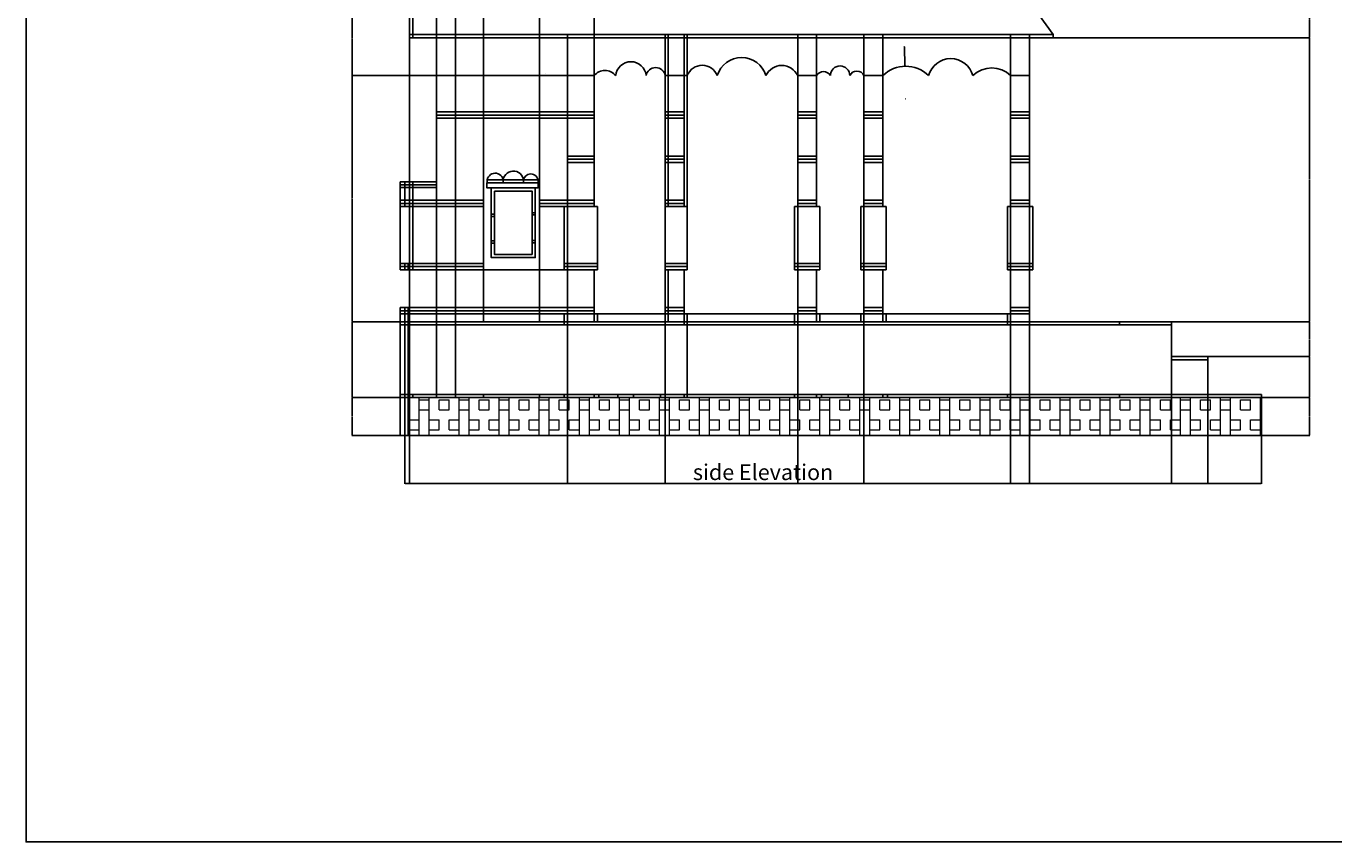
# Model space of a CAD drawing. Units: inches. Extents: x 386 to 107067, y -7 to 96314.
# Tile 1 of 10: x 386 to 1215, y -7 to 510. Entities that reach past the tile are written whole.
import ezdxf

# ---------------------------------------------------------------- set-up
doc = ezdxf.new("R2010")
doc.units = ezdxf.units.IN
for name, color, linetype, lineweight in [('A-ANNO-DIMS', 2, 'Continuous', 18), ('A-ANNO-TEXT', 7, 'Continuous', 25), ('A-ELEV', 7, 'Continuous', 25), ('A-ELEV-PATT', 8, 'Continuous', 13)]:
    doc.layers.add(name, color=color, linetype=linetype, lineweight=lineweight)
doc.styles.get("Standard").update_dxf_attribs({"font": 'arial.ttf'})
doc.dimstyles.get("Standard").update_dxf_attribs({"dimtxt": 0.18, "dimasz": 0.18, "dimexe": 0.18, "dimexo": 0.0625, "dimgap": 0.09, "dimtad": 0, "dimtih": 1, "dimtoh": 1, "dimdec": 4, "dimzin": 0, "dimdsep": 46, "dimtxsty": 'Standard', "dimcen": 0.09, "dimadec": 0, "dimazin": 0, "dimtfac": 1, "dimtdec": 4, "dimtofl": 0, "dimtmove": 0, "dimatfit": 3, "dimfxl": 1, "dimtolj": 1, "dimtzin": 0, "dimarcsym": 0})

# ---------------------------------------------------------------- blocks, each defined once
blk = doc.blocks.new('*D52')
at = {"layer": 'A-ANNO-DIMS', "color": 0, "lineweight": -2, "transparency": 16777216}
for p, q in [((626.03, 250.45), (626.03, 219.83)), ((1169.03, 250.45), (1169.03, 219.83)), ((626.21, 220.01), (897.24, 220.01)), ((1168.85, 220.01), (897.81, 220.01))]:
    blk.add_line(p, q, dxfattribs=at)
at = {"layer": 'A-ANNO-DIMS', "color": 0, "transparency": 16777216}
for points in [[(626.21, 220.04), (626.21, 219.98), (626.03, 220.01)], [(1168.85, 220.04), (1168.85, 219.98), (1169.03, 220.01)]]:
    blk.add_solid(points, dxfattribs=at)
at = {"layer": 'Defpoints', "color": 0, "transparency": 16777216}
for p in [(626.03, 250.51), (1169.03, 250.51), (1169.03, 220.01)]:
    blk.add_point(p, dxfattribs=at)
at = {"layer": 'A-ANNO-DIMS', "color": 0, "transparency": 16777216, "insert": (897.53, 220.01), "char_height": 0.18, "attachment_point": 5}
blk.add_mtext('\\A1;543', dxfattribs=at)
blk = doc.blocks.new('*D53')
at = {"layer": 'A-ANNO-DIMS', "color": 0, "lineweight": -2, "transparency": 16777216}
for p, q in [((622.96, 274.51), (592.35, 274.51)), ((592.53, 274.33), (592.53, 262.69)), ((592.53, 250.69), (592.53, 262.33)), ((622.96, 250.51), (592.35, 250.51))]:
    blk.add_line(p, q, dxfattribs=at)
at = {"layer": 'A-ANNO-DIMS', "color": 0, "transparency": 16777216}
for points in [[(592.5, 274.33), (592.56, 274.33), (592.53, 274.51)], [(592.5, 250.69), (592.56, 250.69), (592.53, 250.51)]]:
    blk.add_solid(points, dxfattribs=at)
at = {"layer": 'Defpoints', "color": 0, "transparency": 16777216}
for p in [(592.53, 274.51), (623.03, 274.51), (623.03, 250.51)]:
    blk.add_point(p, dxfattribs=at)
at = {"layer": 'A-ANNO-DIMS', "color": 0, "transparency": 16777216, "insert": (592.53, 262.51), "char_height": 0.18, "attachment_point": 5}
blk.add_mtext('\\A1;24', dxfattribs=at)
blk = doc.blocks.new('*D54')
at = {"layer": 'A-ANNO-DIMS', "color": 0, "lineweight": -2, "transparency": 16777216}
for p, q in [((622.96, 322.51), (592.35, 322.51)), ((592.53, 322.33), (592.53, 298.69)), ((592.53, 274.69), (592.53, 298.33)), ((622.96, 274.51), (592.35, 274.51))]:
    blk.add_line(p, q, dxfattribs=at)
at = {"layer": 'A-ANNO-DIMS', "color": 0, "transparency": 16777216}
for points in [[(592.5, 322.33), (592.56, 322.33), (592.53, 322.51)], [(592.5, 274.69), (592.56, 274.69), (592.53, 274.51)]]:
    blk.add_solid(points, dxfattribs=at)
at = {"layer": 'Defpoints', "color": 0, "transparency": 16777216}
for p in [(592.53, 322.51), (623.03, 322.51), (623.03, 274.51)]:
    blk.add_point(p, dxfattribs=at)
at = {"layer": 'A-ANNO-DIMS', "color": 0, "transparency": 16777216, "insert": (592.53, 298.51), "char_height": 0.18, "attachment_point": 5}
blk.add_mtext('\\A1;48', dxfattribs=at)
blk = doc.blocks.new('*D55')
at = {"layer": 'A-ANNO-DIMS', "color": 0, "lineweight": -2, "transparency": 16777216}
for p, q in [((728.96, 478.51), (592.35, 478.51)), ((592.53, 478.33), (592.53, 400.69)), ((592.53, 322.69), (592.53, 400.33)), ((622.96, 322.51), (592.35, 322.51))]:
    blk.add_line(p, q, dxfattribs=at)
at = {"layer": 'A-ANNO-DIMS', "color": 0, "transparency": 16777216}
for points in [[(592.5, 478.33), (592.56, 478.33), (592.53, 478.51)], [(592.5, 322.69), (592.56, 322.69), (592.53, 322.51)]]:
    blk.add_solid(points, dxfattribs=at)
at = {"layer": 'Defpoints', "color": 0, "transparency": 16777216}
for p in [(592.53, 478.51), (729.03, 478.51), (623.03, 322.51)]:
    blk.add_point(p, dxfattribs=at)
at = {"layer": 'A-ANNO-DIMS', "color": 0, "transparency": 16777216, "insert": (592.53, 400.51), "char_height": 0.18, "attachment_point": 5}
blk.add_mtext('\\A1;156', dxfattribs=at)
blk = doc.blocks.new('*D56')
at = {"layer": 'A-ANNO-DIMS', "color": 0, "lineweight": -2, "transparency": 16777216}
for p, q in [((628.96, 525.24), (592.35, 525.24)), ((592.53, 525.06), (592.53, 502.06)), ((592.53, 478.69), (592.53, 501.69)), ((728.96, 478.51), (592.35, 478.51))]:
    blk.add_line(p, q, dxfattribs=at)
at = {"layer": 'A-ANNO-DIMS', "color": 0, "transparency": 16777216}
for points in [[(592.5, 525.06), (592.56, 525.06), (592.53, 525.24)], [(592.5, 478.69), (592.56, 478.69), (592.53, 478.51)]]:
    blk.add_solid(points, dxfattribs=at)
at = {"layer": 'Defpoints', "color": 0, "transparency": 16777216}
for p in [(592.53, 525.24), (629.03, 525.24), (729.03, 478.51)]:
    blk.add_point(p, dxfattribs=at)
at = {"layer": 'A-ANNO-DIMS', "color": 0, "transparency": 16777216, "insert": (592.53, 501.88), "char_height": 0.18, "attachment_point": 5}
blk.add_mtext('\\A1;46.73', dxfattribs=at)
blk = doc.blocks.new('*D61')
at = {"layer": 'A-ANNO-DIMS', "color": 0, "lineweight": -2, "transparency": 16777216}
for p, q in [((1169.09, 274.51), (1199.71, 274.51)), ((1199.53, 274.33), (1199.53, 262.69)), ((1199.53, 250.69), (1199.53, 262.33)), ((1169.09, 250.51), (1199.71, 250.51))]:
    blk.add_line(p, q, dxfattribs=at)
at = {"layer": 'A-ANNO-DIMS', "color": 0, "transparency": 16777216}
for points in [[(1199.5, 274.33), (1199.56, 274.33), (1199.53, 274.51)], [(1199.5, 250.69), (1199.56, 250.69), (1199.53, 250.51)]]:
    blk.add_solid(points, dxfattribs=at)
at = {"layer": 'Defpoints', "color": 0, "transparency": 16777216}
for p in [(1169.03, 274.51), (1199.53, 274.51), (1169.03, 250.51)]:
    blk.add_point(p, dxfattribs=at)
at = {"layer": 'A-ANNO-DIMS', "color": 0, "transparency": 16777216, "insert": (1199.53, 262.51), "char_height": 0.18, "attachment_point": 5}
blk.add_mtext('\\A1;24', dxfattribs=at)
blk = doc.blocks.new('*D62')
at = {"layer": 'A-ANNO-DIMS', "color": 0, "lineweight": -2, "transparency": 16777216}
for p, q in [((1135.09, 300.51), (1199.71, 300.51)), ((1199.53, 300.33), (1199.53, 287.69)), ((1199.53, 274.69), (1199.53, 287.33)), ((1135.09, 274.51), (1199.71, 274.51))]:
    blk.add_line(p, q, dxfattribs=at)
at = {"layer": 'A-ANNO-DIMS', "color": 0, "transparency": 16777216}
for points in [[(1199.5, 300.33), (1199.56, 300.33), (1199.53, 300.51)], [(1199.5, 274.69), (1199.56, 274.69), (1199.53, 274.51)]]:
    blk.add_solid(points, dxfattribs=at)
at = {"layer": 'Defpoints', "color": 0, "transparency": 16777216}
for p in [(1135.03, 300.51), (1199.53, 300.51), (1135.03, 274.51)]:
    blk.add_point(p, dxfattribs=at)
at = {"layer": 'A-ANNO-DIMS', "color": 0, "transparency": 16777216, "insert": (1199.53, 287.51), "char_height": 0.18, "attachment_point": 5}
blk.add_mtext('\\A1;26', dxfattribs=at)
blk = doc.blocks.new('*D63')
at = {"layer": 'A-ANNO-DIMS', "color": 0, "lineweight": -2, "transparency": 16777216}
for p, q in [((1112.09, 322.51), (1199.71, 322.51)), ((1199.53, 322.33), (1199.53, 311.69)), ((1199.53, 300.69), (1199.53, 311.33)), ((1112.09, 300.51), (1199.71, 300.51))]:
    blk.add_line(p, q, dxfattribs=at)
at = {"layer": 'A-ANNO-DIMS', "color": 0, "transparency": 16777216}
for points in [[(1199.5, 322.33), (1199.56, 322.33), (1199.53, 322.51)], [(1199.5, 300.69), (1199.56, 300.69), (1199.53, 300.51)]]:
    blk.add_solid(points, dxfattribs=at)
at = {"layer": 'Defpoints', "color": 0, "transparency": 16777216}
for p in [(1112.03, 322.51), (1199.53, 322.51), (1112.03, 300.51)]:
    blk.add_point(p, dxfattribs=at)
at = {"layer": 'A-ANNO-DIMS', "color": 0, "transparency": 16777216, "insert": (1199.53, 311.51), "char_height": 0.18, "attachment_point": 5}
blk.add_mtext('\\A1;22', dxfattribs=at)
blk = doc.blocks.new('*D64')
at = {"layer": 'A-ANNO-DIMS', "color": 0, "lineweight": -2, "transparency": 16777216}
for p, q in [((1037.1, 502.51), (1199.71, 502.51)), ((1199.53, 502.33), (1199.53, 412.69)), ((1199.53, 322.69), (1199.53, 412.33)), ((1112.09, 322.51), (1199.71, 322.51))]:
    blk.add_line(p, q, dxfattribs=at)
at = {"layer": 'A-ANNO-DIMS', "color": 0, "transparency": 16777216}
for points in [[(1199.5, 502.33), (1199.56, 502.33), (1199.53, 502.51)], [(1199.5, 322.69), (1199.56, 322.69), (1199.53, 322.51)]]:
    blk.add_solid(points, dxfattribs=at)
at = {"layer": 'Defpoints', "color": 0, "transparency": 16777216}
for p in [(1037.04, 502.51), (1199.53, 502.51), (1112.03, 322.51)]:
    blk.add_point(p, dxfattribs=at)
at = {"layer": 'A-ANNO-DIMS', "color": 0, "transparency": 16777216, "insert": (1199.53, 412.51), "char_height": 0.18, "attachment_point": 5}
blk.add_mtext('\\A1;180', dxfattribs=at)
blk = doc.blocks.new('*D65')
at = {"layer": 'A-ANNO-DIMS', "color": 0, "lineweight": -2, "transparency": 16777216}
for p, q in [((1022.09, 525.24), (1199.71, 525.24)), ((1199.53, 525.06), (1199.53, 514.06)), ((1199.53, 502.69), (1199.53, 513.69)), ((1037.1, 502.51), (1199.71, 502.51))]:
    blk.add_line(p, q, dxfattribs=at)
at = {"layer": 'A-ANNO-DIMS', "color": 0, "transparency": 16777216}
for points in [[(1199.5, 525.06), (1199.56, 525.06), (1199.53, 525.24)], [(1199.5, 502.69), (1199.56, 502.69), (1199.53, 502.51)]]:
    blk.add_solid(points, dxfattribs=at)
at = {"layer": 'Defpoints', "color": 0, "transparency": 16777216}
for p in [(1022.03, 525.24), (1199.53, 525.24), (1037.04, 502.51)]:
    blk.add_point(p, dxfattribs=at)
at = {"layer": 'A-ANNO-DIMS', "color": 0, "transparency": 16777216, "insert": (1199.53, 513.88), "char_height": 0.18, "attachment_point": 5}
blk.add_mtext('\\A1;22.735', dxfattribs=at)
blk = doc.blocks.new('*D68')
at = {"layer": 'A-ANNO-DIMS', "color": 0, "lineweight": -2, "transparency": 16777216}
for p, q in [((629.03, 502.45), (629.03, 219.83)), ((729.03, 504.45), (729.03, 219.83)), ((629.21, 220.01), (678.75, 220.01)), ((728.85, 220.01), (679.31, 220.01))]:
    blk.add_line(p, q, dxfattribs=at)
at = {"layer": 'A-ANNO-DIMS', "color": 0, "transparency": 16777216}
for points in [[(629.21, 220.04), (629.21, 219.98), (629.03, 220.01)], [(728.85, 220.04), (728.85, 219.98), (729.03, 220.01)]]:
    blk.add_solid(points, dxfattribs=at)
at = {"layer": 'Defpoints', "color": 0, "transparency": 16777216}
for p in [(629.03, 502.51), (729.03, 504.51), (729.03, 220.01)]:
    blk.add_point(p, dxfattribs=at)
at = {"layer": 'A-ANNO-DIMS', "color": 0, "transparency": 16777216, "insert": (679.03, 220.01), "char_height": 0.18, "attachment_point": 5}
blk.add_mtext('\\A1;100', dxfattribs=at)
blk = doc.blocks.new('*D69')
at = {"layer": 'A-ANNO-DIMS', "color": 0, "lineweight": -2, "transparency": 16777216}
for p, q in [((729.03, 504.45), (729.03, 219.83)), ((791.03, 504.45), (791.03, 219.83)), ((729.21, 220.01), (759.81, 220.01)), ((790.85, 220.01), (760.24, 220.01))]:
    blk.add_line(p, q, dxfattribs=at)
at = {"layer": 'A-ANNO-DIMS', "color": 0, "transparency": 16777216}
for points in [[(729.21, 220.04), (729.21, 219.98), (729.03, 220.01)], [(790.85, 220.04), (790.85, 219.98), (791.03, 220.01)]]:
    blk.add_solid(points, dxfattribs=at)
at = {"layer": 'Defpoints', "color": 0, "transparency": 16777216}
for p in [(729.03, 504.51), (791.03, 504.51), (791.03, 220.01)]:
    blk.add_point(p, dxfattribs=at)
at = {"layer": 'A-ANNO-DIMS', "color": 0, "transparency": 16777216, "insert": (760.03, 220.01), "char_height": 0.18, "attachment_point": 5}
blk.add_mtext('\\A1;62', dxfattribs=at)
blk = doc.blocks.new('*D70')
at = {"layer": 'A-ANNO-DIMS', "color": 0, "lineweight": -2, "transparency": 16777216}
for p, q in [((791.03, 504.45), (791.03, 219.83)), ((875.03, 504.45), (875.03, 219.83)), ((791.21, 220.01), (832.81, 220.01)), ((874.85, 220.01), (833.24, 220.01))]:
    blk.add_line(p, q, dxfattribs=at)
at = {"layer": 'A-ANNO-DIMS', "color": 0, "transparency": 16777216}
for points in [[(791.21, 220.04), (791.21, 219.98), (791.03, 220.01)], [(874.85, 220.04), (874.85, 219.98), (875.03, 220.01)]]:
    blk.add_solid(points, dxfattribs=at)
at = {"layer": 'Defpoints', "color": 0, "transparency": 16777216}
for p in [(791.03, 504.51), (875.03, 504.51), (875.03, 220.01)]:
    blk.add_point(p, dxfattribs=at)
at = {"layer": 'A-ANNO-DIMS', "color": 0, "transparency": 16777216, "insert": (833.03, 220.01), "char_height": 0.18, "attachment_point": 5}
blk.add_mtext('\\A1;84', dxfattribs=at)
blk = doc.blocks.new('*D71')
at = {"layer": 'A-ANNO-DIMS', "color": 0, "lineweight": -2, "transparency": 16777216}
for p, q in [((875.03, 504.45), (875.03, 219.83)), ((917.03, 504.45), (917.03, 219.83)), ((875.21, 220.01), (895.8, 220.01)), ((916.85, 220.01), (896.25, 220.01))]:
    blk.add_line(p, q, dxfattribs=at)
at = {"layer": 'A-ANNO-DIMS', "color": 0, "transparency": 16777216}
for points in [[(875.21, 220.04), (875.21, 219.98), (875.03, 220.01)], [(916.85, 220.04), (916.85, 219.98), (917.03, 220.01)]]:
    blk.add_solid(points, dxfattribs=at)
at = {"layer": 'Defpoints', "color": 0, "transparency": 16777216}
for p in [(875.03, 504.51), (917.03, 504.51), (917.03, 220.01)]:
    blk.add_point(p, dxfattribs=at)
at = {"layer": 'A-ANNO-DIMS', "color": 0, "transparency": 16777216, "insert": (896.03, 220.01), "char_height": 0.18, "attachment_point": 5}
blk.add_mtext('\\A1;42', dxfattribs=at)
blk = doc.blocks.new('*D72')
at = {"layer": 'A-ANNO-DIMS', "color": 0, "lineweight": -2, "transparency": 16777216}
for p, q in [((917.03, 504.45), (917.03, 219.83)), ((1010.03, 504.45), (1010.03, 219.83)), ((917.21, 220.01), (963.31, 220.01)), ((1009.85, 220.01), (963.74, 220.01))]:
    blk.add_line(p, q, dxfattribs=at)
at = {"layer": 'A-ANNO-DIMS', "color": 0, "transparency": 16777216}
for points in [[(917.21, 220.04), (917.21, 219.98), (917.03, 220.01)], [(1009.85, 220.04), (1009.85, 219.98), (1010.03, 220.01)]]:
    blk.add_solid(points, dxfattribs=at)
at = {"layer": 'Defpoints', "color": 0, "transparency": 16777216}
for p in [(917.03, 504.51), (1010.03, 504.51), (1010.03, 220.01)]:
    blk.add_point(p, dxfattribs=at)
at = {"layer": 'A-ANNO-DIMS', "color": 0, "transparency": 16777216, "insert": (963.53, 220.01), "char_height": 0.18, "attachment_point": 5}
blk.add_mtext('\\A1;93', dxfattribs=at)
blk = doc.blocks.new('*D73')
at = {"layer": 'A-ANNO-DIMS', "color": 0, "lineweight": -2, "transparency": 16777216}
for p, q in [((1010.03, 504.45), (1010.03, 219.83)), ((1022.03, 502.45), (1022.03, 219.83)), ((1010.21, 220.01), (1015.82, 220.01)), ((1021.85, 220.01), (1016.23, 220.01))]:
    blk.add_line(p, q, dxfattribs=at)
at = {"layer": 'A-ANNO-DIMS', "color": 0, "transparency": 16777216}
for points in [[(1010.21, 220.04), (1010.21, 219.98), (1010.03, 220.01)], [(1021.85, 220.04), (1021.85, 219.98), (1022.03, 220.01)]]:
    blk.add_solid(points, dxfattribs=at)
at = {"layer": 'Defpoints', "color": 0, "transparency": 16777216}
for p in [(1010.03, 504.51), (1022.03, 502.51), (1022.03, 220.01)]:
    blk.add_point(p, dxfattribs=at)
at = {"layer": 'A-ANNO-DIMS', "color": 0, "transparency": 16777216, "insert": (1016.03, 220.01), "char_height": 0.18, "attachment_point": 5}
blk.add_mtext('\\A1;12', dxfattribs=at)
blk = doc.blocks.new('*D74')
at = {"layer": 'A-ANNO-DIMS', "color": 0, "lineweight": -2, "transparency": 16777216}
for p, q in [((1022.03, 322.45), (1022.03, 219.83)), ((1112.03, 322.45), (1112.03, 219.83)), ((1022.21, 220.01), (1066.81, 220.01)), ((1111.85, 220.01), (1067.24, 220.01))]:
    blk.add_line(p, q, dxfattribs=at)
at = {"layer": 'A-ANNO-DIMS', "color": 0, "transparency": 16777216}
for points in [[(1022.21, 220.04), (1022.21, 219.98), (1022.03, 220.01)], [(1111.85, 220.04), (1111.85, 219.98), (1112.03, 220.01)]]:
    blk.add_solid(points, dxfattribs=at)
at = {"layer": 'Defpoints', "color": 0, "transparency": 16777216}
for p in [(1022.03, 322.51), (1112.03, 322.51), (1112.03, 220.01)]:
    blk.add_point(p, dxfattribs=at)
at = {"layer": 'A-ANNO-DIMS', "color": 0, "transparency": 16777216, "insert": (1067.03, 220.01), "char_height": 0.18, "attachment_point": 5}
blk.add_mtext('\\A1;90', dxfattribs=at)
blk = doc.blocks.new('*D75')
at = {"layer": 'A-ANNO-DIMS', "color": 0, "lineweight": -2, "transparency": 16777216}
for p, q in [((1112.03, 300.45), (1112.03, 219.83)), ((1135.03, 300.45), (1135.03, 219.83)), ((1112.21, 220.01), (1123.3, 220.01)), ((1134.85, 220.01), (1123.75, 220.01))]:
    blk.add_line(p, q, dxfattribs=at)
at = {"layer": 'A-ANNO-DIMS', "color": 0, "transparency": 16777216}
for points in [[(1112.21, 220.04), (1112.21, 219.98), (1112.03, 220.01)], [(1134.85, 220.04), (1134.85, 219.98), (1135.03, 220.01)]]:
    blk.add_solid(points, dxfattribs=at)
at = {"layer": 'Defpoints', "color": 0, "transparency": 16777216}
for p in [(1112.03, 300.51), (1135.03, 300.51), (1135.03, 220.01)]:
    blk.add_point(p, dxfattribs=at)
at = {"layer": 'A-ANNO-DIMS', "color": 0, "transparency": 16777216, "insert": (1123.53, 220.01), "char_height": 0.18, "attachment_point": 5}
blk.add_mtext('\\A1;23', dxfattribs=at)
blk = doc.blocks.new('*D76')
at = {"layer": 'A-ANNO-DIMS', "color": 0, "lineweight": -2, "transparency": 16777216}
for p, q in [((1135.03, 274.45), (1135.03, 219.83)), ((1169.03, 274.45), (1169.03, 219.83)), ((1135.21, 220.01), (1151.81, 220.01)), ((1168.85, 220.01), (1152.24, 220.01))]:
    blk.add_line(p, q, dxfattribs=at)
at = {"layer": 'A-ANNO-DIMS', "color": 0, "transparency": 16777216}
for points in [[(1135.21, 220.04), (1135.21, 219.98), (1135.03, 220.01)], [(1168.85, 220.04), (1168.85, 219.98), (1169.03, 220.01)]]:
    blk.add_solid(points, dxfattribs=at)
at = {"layer": 'Defpoints', "color": 0, "transparency": 16777216}
for p in [(1135.03, 274.51), (1169.03, 274.51), (1169.03, 220.01)]:
    blk.add_point(p, dxfattribs=at)
at = {"layer": 'A-ANNO-DIMS', "color": 0, "transparency": 16777216, "insert": (1152.03, 220.01), "char_height": 0.18, "attachment_point": 5}
blk.add_mtext('\\A1;34', dxfattribs=at)
blk = doc.blocks.new('*D91')
at = {"layer": 'A-ANNO-DIMS', "color": 0, "lineweight": -2, "transparency": 16777216}
for p, q in [((942.49, 496.82), (942.67, 496.82)), ((942.67, 496.82), (942.98, 484.63)), ((943.42, 463.83), (943.6, 463.83)), ((943.51, 463.74), (943.51, 463.92))]:
    blk.add_line(p, q, dxfattribs=at)
at = {"layer": 'A-ANNO-DIMS', "color": 0, "transparency": 16777216}
blk.add_solid([(943.01, 484.63), (942.95, 484.63), (942.99, 484.45)], dxfattribs=at)
at = {"layer": 'Defpoints', "color": 0, "transparency": 16777216}
for p in [(942.99, 484.45), (943.51, 463.83)]:
    blk.add_point(p, dxfattribs=at)
at = {"layer": 'A-ANNO-DIMS', "color": 0, "transparency": 16777216, "insert": (941.94, 496.82), "char_height": 0.18, "attachment_point": 5}
blk.add_mtext('\\A1;R20.624', dxfattribs=at)

msp = doc.modelspace()

# ---------------------------------------------------------------- hatches: boundary and pattern name
at = {"layer": 'A-ELEV-PATT'}
h = msp.add_hatch(dxfattribs=at)
h.set_pattern_fill('BOX', color=256)
h.paths.add_polyline_path([(1169.0252, 274.5096), (628.0252, 274.5096), (628.0252, 250.5096), (1169.0252, 250.5096)])

# ---------------------------------------------------------------- linework, layer by layer
at = {"layer": 'A-ELEV'}
for p, q in [((675.7732, 612.7565), (675.7732, 451.5096)), ((711.2692, 612.7565), (711.2692, 322.5096)), ((646.0252, 593.3749), (646.0252, 274.5096)), ((629.0252, 585.7146), (629.0252, 502.5096)), ((629.0252, 585.7146), (629.0252, 502.5096)), ((631.0252, 585.7146), (631.0252, 502.5096)), ((658.0252, 525.2442), (658.0252, 274.5096)), ((746.0252, 525.2442), (746.0252, 395.5096)), ((1037.0367, 504.5096), (1022.0252, 525.2442)), ((1022.0252, 504.5096), (629.0252, 504.5096)), ((1022.0252, 502.5096), (629.0252, 502.5096)), ((729.0252, 504.5096), (729.0252, 395.5096)), ((791.0252, 504.5096), (791.0252, 355.5096)), ((793.0252, 504.5096), (793.0252, 395.5096)), ((803.0252, 504.5096), (803.0252, 395.5096)), ((805.0252, 504.5096), (805.0252, 355.5096)), ((875.0252, 504.5096), (875.0252, 395.5096)), ((887.0252, 504.5096), (887.0252, 395.5096)), ((917.0252, 504.5096), (917.0252, 395.5096)), ((929.0252, 504.5096), (929.0252, 395.5096)), ((1010.0252, 504.5096), (1010.0252, 395.5096)), ((1022.0252, 501.2442), (1022.0252, 504.5096)), ((1022.0252, 504.5096), (1037.0367, 504.5096)), ((1022.0252, 504.5096), (1022.0252, 395.5096)), ((1022.0252, 478.5096), (1022.0252, 502.5096)), ((1022.0252, 502.5096), (1036.8733, 502.5096)), ((1037.0367, 504.5096), (1037.0367, 502.5096)), ((715.3564, 479.848), (715.3564, 479.848)), ((729.0252, 479.848), (729.0252, 478.5096)), ((746.0252, 478.5096), (729.0252, 478.5096)), ((805.0252, 478.5096), (791.0252, 478.5096)), ((887.0252, 478.5096), (875.0252, 478.5096)), ((929.0252, 478.5096), (917.0252, 478.5096)), ((1022.0252, 478.5096), (1010.0252, 478.5096)), ((1022.0252, 395.5096), (1022.0252, 478.5096)), ((746.0252, 455.5096), (646.0252, 455.5096)), ((746.0252, 453.5096), (646.0252, 453.5096)), ((746.0252, 451.5096), (646.0252, 451.5096)), ((675.7732, 451.5096), (675.7732, 322.5096)), ((803.0252, 455.5096), (791.0252, 455.5096)), ((803.0252, 453.5096), (791.0252, 453.5096)), ((803.0252, 451.5096), (791.0252, 451.5096)), ((887.0252, 455.5096), (875.0252, 455.5096)), ((887.0252, 453.5096), (875.0252, 453.5096)), ((887.0252, 451.5096), (875.0252, 451.5096)), ((929.0252, 455.5096), (917.0252, 455.5096)), ((929.0252, 453.5096), (917.0252, 453.5096)), ((929.0252, 451.5096), (917.0252, 451.5096)), ((1022.0252, 455.5096), (1010.0252, 455.5096)), ((1022.0252, 453.5096), (1010.0252, 453.5096)), ((1022.0252, 451.5096), (1010.0252, 451.5096)), ((746.0252, 427.5096), (729.0252, 427.5096)), ((746.0252, 425.5096), (729.0252, 425.5096)), ((746.0252, 423.5096), (729.0252, 423.5096)), ((803.0252, 427.5096), (791.0252, 427.5096)), ((803.0252, 425.5096), (791.0252, 425.5096)), ((803.0252, 423.5096), (791.0252, 423.5096)), ((887.0252, 427.5096), (875.0252, 427.5096)), ((887.0252, 425.5096), (875.0252, 425.5096)), ((887.0252, 423.5096), (875.0252, 423.5096)), ((929.0252, 427.5096), (917.0252, 427.5096)), ((929.0252, 425.5096), (917.0252, 425.5096)), ((929.0252, 423.5096), (917.0252, 423.5096)), ((1022.0252, 427.5096), (1010.0252, 427.5096)), ((1022.0252, 425.5096), (1010.0252, 425.5096)), ((1022.0252, 423.5096), (1010.0252, 423.5096)), ((623.0252, 411.1778), (623.0252, 355.5096)), ((623.0252, 411.1778), (623.0252, 355.5096)), ((646.0252, 411.1778), (623.0252, 411.1778)), ((623.0252, 409.3312), (646.0252, 409.3312)), ((623.0252, 407.5372), (646.0252, 407.5372)), ((626.0252, 411.1778), (626.0252, 395.5096)), ((629.0252, 407.5372), (629.0252, 411.1778)), ((629.0252, 411.1778), (629.0252, 355.5096)), ((629.0252, 411.1778), (629.0252, 355.5096)), ((631.0252, 411.1778), (631.0252, 355.5096)), ((675.7732, 399.5096), (623.0252, 399.5096)), ((746.0252, 399.5096), (711.2692, 399.5096)), ((803.0252, 399.5096), (791.0252, 399.5096)), ((887.0252, 399.5096), (875.0252, 399.5096)), ((929.0252, 399.5096), (917.0252, 399.5096)), ((1022.0252, 399.5096), (1010.0252, 399.5096)), ((675.7732, 397.5096), (623.0252, 397.5096)), ((629.0252, 395.5096), (623.0252, 395.5096)), ((675.7732, 395.5096), (623.0252, 395.5096)), ((682.7356, 390.8156), (680.7356, 390.8156)), ((708.6415, 391.4912), (706.6415, 391.4912)), ((708.6415, 390.2151), (706.6415, 390.2151)), ((746.0252, 397.5096), (711.2692, 397.5096)), ((748.0252, 395.5096), (711.2692, 395.5096)), ((727.0252, 395.5096), (727.0252, 355.5096)), ((746.0252, 395.5096), (729.0252, 395.5096)), ((748.0252, 395.5096), (748.0252, 355.5096)), ((803.0252, 397.5096), (791.0252, 397.5096)), ((803.0252, 395.5096), (791.0252, 395.5096)), ((805.0252, 395.5096), (791.0252, 395.5096)), ((873.0252, 395.5096), (873.0252, 355.5096)), ((889.0252, 395.5096), (873.0252, 395.5096)), ((887.0252, 397.5096), (875.0252, 397.5096)), ((887.0252, 395.5096), (875.0252, 395.5096)), ((889.0252, 395.5096), (889.0252, 355.5096)), ((915.0252, 395.5096), (915.0252, 355.5096)), ((931.0252, 395.5096), (915.0252, 395.5096)), ((929.0252, 397.5096), (917.0252, 397.5096)), ((929.0252, 395.5096), (917.0252, 395.5096)), ((931.0252, 395.5096), (931.0252, 355.5096)), ((1008.0252, 395.5096), (1008.0252, 355.5096)), ((1024.0252, 395.5096), (1008.0252, 395.5096)), ((1022.0252, 397.5096), (1010.0252, 397.5096)), ((1022.0252, 395.5096), (1010.0252, 395.5096)), ((1024.0252, 355.5096), (1024.0252, 395.5096)), ((682.7356, 389.3143), (680.7356, 389.3143)), ((682.7356, 373.9258), (680.7356, 373.9258)), ((708.6415, 374.0009), (706.6415, 374.0009)), ((682.7356, 372.4245), (680.7356, 372.4245)), ((708.6415, 372.5746), (706.6415, 372.5746)), ((675.7732, 359.5096), (623.0252, 359.5096)), ((675.7732, 357.5096), (623.0252, 357.5096)), ((626.0252, 359.5096), (626.0252, 355.5096)), ((628.0252, 359.5096), (628.0252, 355.5096)), ((748.0252, 359.5096), (727.0252, 359.5096)), ((748.0252, 357.5096), (727.0252, 357.5096)), ((805.0252, 359.5096), (791.0252, 359.5096)), ((805.0252, 357.5096), (791.0252, 357.5096)), ((889.0252, 359.5096), (873.0252, 359.5096)), ((889.0252, 357.5096), (873.0252, 357.5096)), ((931.0252, 359.5096), (915.0252, 359.5096)), ((931.0252, 357.5096), (915.0252, 357.5096)), ((1024.0252, 359.5096), (1008.0252, 359.5096)), ((1024.0252, 357.5096), (1008.0252, 357.5096)), ((629.0252, 355.5096), (623.0252, 355.5096)), ((748.0252, 355.5096), (623.0252, 355.5096)), ((746.0252, 355.5096), (729.0252, 355.5096)), ((729.0252, 355.5096), (729.0252, 274.5096)), ((746.0252, 355.5096), (746.0252, 322.5096)), ((803.0252, 355.5096), (791.0252, 355.5096)), ((805.0252, 355.5096), (791.0252, 355.5096)), ((793.0252, 355.5096), (793.0252, 322.5096)), ((803.0252, 355.5096), (803.0252, 320.5096)), ((889.0252, 355.5096), (873.0252, 355.5096)), ((887.0252, 355.5096), (875.0252, 355.5096)), ((875.0252, 355.5096), (875.0252, 274.5096)), ((887.0252, 355.5096), (887.0252, 322.5096)), ((931.0252, 355.5096), (915.0252, 355.5096)), ((929.0252, 355.5096), (917.0252, 355.5096)), ((917.0252, 355.5096), (917.0252, 322.5096)), ((929.0252, 355.5096), (929.0252, 322.5096)), ((1024.0252, 355.5096), (1008.0252, 355.5096)), ((1022.0252, 355.5096), (1010.0252, 355.5096)), ((1010.0252, 355.5096), (1010.0252, 274.5096)), ((1022.0252, 322.5096), (1022.0252, 355.5096)), ((1022.0252, 355.5096), (1022.0252, 274.5096)), ((629.0252, 331.5096), (623.0252, 331.5096)), ((623.0252, 331.5096), (623.0252, 250.5096)), ((623.0252, 331.5096), (623.0252, 250.5096)), ((629.0252, 329.5096), (623.0252, 329.5096)), ((1022.0252, 327.5096), (623.0252, 327.5096)), ((626.0252, 331.5096), (626.0252, 250.5096)), ((628.0252, 331.5096), (628.0252, 250.5096)), ((746.0252, 331.5096), (629.0252, 331.5096)), ((746.0252, 329.5096), (629.0252, 329.5096)), ((727.0252, 327.5096), (727.0252, 320.5096)), ((748.0252, 327.5096), (748.0252, 322.5096)), ((803.0252, 331.5096), (791.0252, 331.5096)), ((791.0252, 331.5096), (791.0252, 322.5096)), ((803.0252, 329.5096), (791.0252, 329.5096)), ((805.0252, 327.5096), (805.0252, 274.5096)), ((873.0252, 327.5096), (873.0252, 320.5096)), ((887.0252, 331.5096), (875.0252, 331.5096)), ((887.0252, 329.5096), (875.0252, 329.5096)), ((889.0252, 327.5096), (889.0252, 322.5096)), ((915.0252, 327.5096), (915.0252, 322.5096)), ((929.0252, 331.5096), (917.0252, 331.5096)), ((929.0252, 329.5096), (917.0252, 329.5096)), ((931.0252, 327.5096), (931.0252, 322.5096)), ((1008.0252, 327.5096), (1008.0252, 320.5096)), ((1022.0252, 331.5096), (1010.0252, 331.5096)), ((1022.0252, 329.5096), (1010.0252, 329.5096)), ((1022.0252, 322.5096), (1022.0252, 327.5096)), ((623.0252, 322.5096), (1112.0252, 322.5096)), ((623.0252, 320.5096), (1112.0252, 320.5096)), ((1079.0252, 322.5096), (1079.0252, 320.5096)), ((1112.0252, 322.5096), (1112.0252, 274.5096)), ((1135.0252, 300.5096), (1112.0252, 300.5096)), ((1135.0252, 298.5096), (1112.0252, 298.5096)), ((1135.0252, 300.5096), (1135.0252, 298.5096)), ((1135.0252, 298.5096), (1135.0252, 274.5096)), ((623.0252, 276.5096), (1169.0252, 276.5096)), ((623.0252, 274.5096), (1169.0252, 274.5096)), ((629.0252, 276.5096), (629.0252, 274.5096)), ((629.0252, 276.5096), (629.0252, 274.5096)), ((631.0252, 276.5096), (631.0252, 274.5096)), ((675.7732, 276.5096), (675.7732, 274.5096)), ((711.2692, 276.5096), (711.2692, 274.5096)), ((727.0252, 276.5096), (727.0252, 274.5096)), ((746.0252, 276.5096), (746.0252, 274.5096)), ((749.0252, 276.5096), (749.0252, 274.5096)), ((761.0252, 276.5096), (761.0252, 274.5096)), ((771.0252, 276.5096), (771.0252, 274.5096)), ((788.0252, 276.5096), (788.0252, 274.5096)), ((791.0252, 276.5096), (791.0252, 274.5096)), ((803.0252, 276.5096), (803.0252, 274.5096)), ((873.0252, 276.5096), (873.0252, 274.5096)), ((887.0252, 276.5096), (887.0252, 274.5096)), ((890.0252, 276.5096), (890.0252, 274.5096)), ((907.0252, 276.5096), (907.0252, 274.5096)), ((917.0252, 276.5096), (917.0252, 274.5096)), ((929.0252, 276.5096), (929.0252, 274.5096)), ((932.0252, 276.5096), (932.0252, 274.5096)), ((1008.0252, 276.5096), (1008.0252, 274.5096)), ((1079.0252, 276.5096), (1079.0252, 274.5096)), ((1169.0252, 276.5096), (1169.0252, 250.5096)), ((623.0252, 250.5096), (1169.0252, 250.5096))]:
    msp.add_line(p, q, dxfattribs=at)
for points in [[(385.946, 1737.774), (1886.0535, 1737.774), (1886.0535, -7.0679), (385.946, -7.0679)], [(678.0385, 410.674), (710.4326, 410.674), (710.4326, 407.4116), (678.0385, 407.4116)], [(678.2042, 412.4395), (710.4326, 412.4395), (710.4326, 410.674), (678.2042, 410.674)], [(680.7356, 407.3359), (708.6415, 407.3359), (708.6415, 363.2224), (680.7356, 363.2224)], [(682.7356, 405.3359), (706.6415, 405.3359), (706.6415, 365.2224), (682.7356, 365.2224)]]:
    msp.add_lwpolyline(points, close=True, dxfattribs=at)
for centre, radius, start, end in [((839.4626, 473.8743), 16.0952, 16.7377051, 163.2622949), ((972.0541, 474.7532), 14.5469, 14.9650391, 165.0349609), ((752.834, 473.2537), 8.6014, 37.6655602, 142.3344398), ((769.3202, 477.653), 9.7152, 5.0587521, 174.9412479), ((785.0114, 477.5629), 6.0879, 8.9462473, 171.0537527), ((814.5372, 474.8721), 10.1838, 20.9273808, 159.0726192), ((864.9506, 473.8743), 11.0898, 24.7069227, 155.2930773), ((891.3873, 476.127), 4.9704, 28.6436161, 151.3563839), ((901.9146, 478.5096), 6.1652, 0, 180), ((912.5525, 476.5833), 4.8699, 23.3003483, 156.6996365), ((943.5129, 463.8305), 20.6245, 45.3759646, 134.6240354), ((998.0664, 466.4446), 16.9876, 45.2533905, 134.7466095), ((683.2677, 411.5567), 5.1399, 350.1110871, 170.1110871), ((694.7953, 411.5567), 6.524, 352.2238795, 172.2238795), ((705.846, 411.5567), 4.6708, 349.1063041, 169.1063041)]:
    msp.add_arc(centre, radius, start, end, dxfattribs=at)

# ---------------------------------------------------------------- texts
at = {"layer": 'A-ANNO-TEXT', "insert": (808.6098, 232.1989), "char_height": 10, "attachment_point": 1}
msp.add_mtext_dynamic_manual_height_columns('side Elevation', width=177.910198, gutter_width=12.5, heights=[0], dxfattribs=at)

# ---------------------------------------------------------------- dimensions: what is measured, and where the dimension line sits
at = {"layer": 'A-ANNO-DIMS'}
for base, p1, p2, override, picture, middle in [((592.5252, 525.2442), (729.0252, 478.5096), (629.0252, 525.2442), {"dimdec": 2, "dimlfac": 1, "dimrnd": 0, "dimzin": 0, "dimdsep": 46, "dimlunit": 2}, '*D56', (592.5252, 501.8769)), ((1199.5252, 525.2442), (1037.0367, 502.5096), (1022.0252, 525.2442), {"dimdec": 3, "dimlfac": 1, "dimrnd": 0, "dimzin": 0, "dimdsep": 46, "dimlunit": 2}, '*D65', (1199.5252, 513.8769)), ((1199.5252, 502.5096), (1112.0252, 322.5096), (1037.0367, 502.5096), {"dimdec": 0, "dimlfac": 1, "dimrnd": 0, "dimzin": 0, "dimdsep": 46, "dimlunit": 2}, '*D64', (1199.5252, 412.5096)), ((592.5252, 478.5096), (623.0252, 322.5096), (729.0252, 478.5096), {"dimdec": 0, "dimlfac": 1, "dimrnd": 0, "dimzin": 0, "dimdsep": 46, "dimlunit": 2}, '*D55', (592.5252, 400.5096)), ((592.5252, 322.5096), (623.0252, 274.5096), (623.0252, 322.5096), {"dimdec": 0, "dimlfac": 1, "dimrnd": 0, "dimzin": 0, "dimdsep": 46, "dimlunit": 2}, '*D54', (592.5252, 298.5096)), ((1199.5252, 322.5096), (1112.0252, 300.5096), (1112.0252, 322.5096), {"dimdec": 0, "dimlfac": 1, "dimrnd": 0, "dimzin": 0, "dimdsep": 46, "dimlunit": 2}, '*D63', (1199.5252, 311.5096)), ((1199.5252, 300.5096), (1135.0252, 274.5096), (1135.0252, 300.5096), {"dimdec": 0, "dimlfac": 1, "dimrnd": 0, "dimzin": 0, "dimdsep": 46, "dimlunit": 2}, '*D62', (1199.5252, 287.5096)), ((592.5252, 274.5096), (623.0252, 250.5096), (623.0252, 274.5096), {"dimdec": 0, "dimlfac": 1, "dimrnd": 0, "dimzin": 0, "dimdsep": 46, "dimlunit": 2}, '*D53', (592.5252, 262.5096)), ((1199.5252, 274.5096), (1169.0252, 250.5096), (1169.0252, 274.5096), {"dimdec": 0, "dimlfac": 1, "dimrnd": 0, "dimzin": 0, "dimdsep": 46, "dimlunit": 2}, '*D61', (1199.5252, 262.5096))]:
    dim = msp.add_linear_dim(base=base, p1=p1, p2=p2, angle=90, dimstyle='Standard', override=override, dxfattribs=at)
    dim.commit()
    dim.dimension.update_dxf_attribs({"geometry": picture, "text_midpoint": middle})
for base, p1, p2, picture, middle in [((729.0252, 220.0096), (629.0252, 502.5096), (729.0252, 504.5096), '*D68', (679.0252, 220.0096)), ((791.0252, 220.0096), (729.0252, 504.5096), (791.0252, 504.5096), '*D69', (760.0252, 220.0096)), ((875.0252, 220.0096), (791.0252, 504.5096), (875.0252, 504.5096), '*D70', (833.0252, 220.0096)), ((917.0252, 220.0096), (875.0252, 504.5096), (917.0252, 504.5096), '*D71', (896.0252, 220.0096)), ((1010.0252, 220.0096), (917.0252, 504.5096), (1010.0252, 504.5096), '*D72', (963.5252, 220.0096)), ((1022.0252, 220.0096), (1010.0252, 504.5096), (1022.0252, 502.5096), '*D73', (1016.0252, 220.0096)), ((1112.0252, 220.0096), (1022.0252, 322.5096), (1112.0252, 322.5096), '*D74', (1067.0252, 220.0096)), ((1135.0252, 220.0096), (1112.0252, 300.5096), (1135.0252, 300.5096), '*D75', (1123.5252, 220.0096)), ((1169.0252, 220.0096), (1135.0252, 274.5096), (1169.0252, 274.5096), '*D76', (1152.0252, 220.0096)), ((1169.0252, 220.0096), (626.0252, 250.5096), (1169.0252, 250.5096), '*D52', (897.5252, 220.0096))]:
    dim = msp.add_linear_dim(base=base, p1=p1, p2=p2, dimstyle='Standard', override={"dimdec": 0, "dimlfac": 1, "dimrnd": 0, "dimzin": 0, "dimdsep": 46, "dimlunit": 2}, dxfattribs=at)
    dim.commit()
    dim.dimension.update_dxf_attribs({"geometry": picture, "text_midpoint": middle})
dim = msp.add_radius_dim(center=(943.5129, 463.83053), mpoint=(942.9886, 484.44835), dimstyle='Standard', override={"dimdec": 3, "dimlfac": 1, "dimrnd": 0, "dimzin": 0, "dimdsep": 46, "dimlunit": 2}, dxfattribs=at)
dim.commit()
dim.dimension.update_dxf_attribs({"geometry": '*D91', "text_midpoint": (941.94462, 496.81905), "dimtype": 164})

doc.saveas('drawing.dxf')
